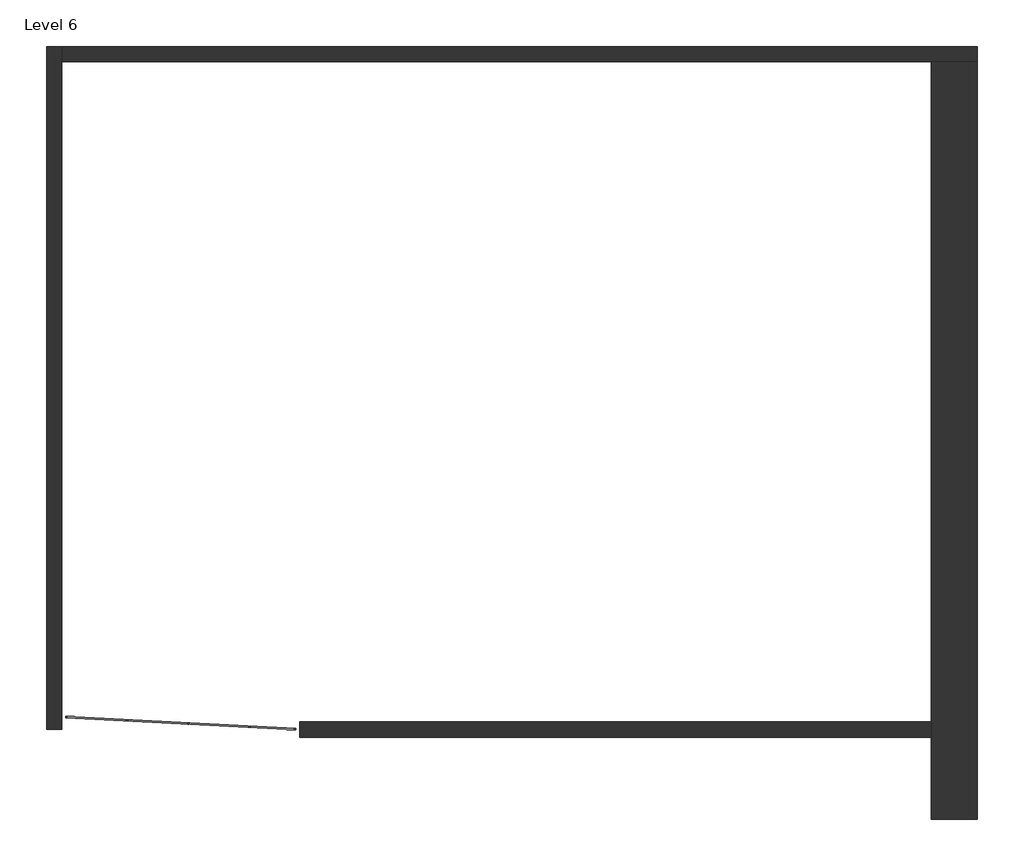
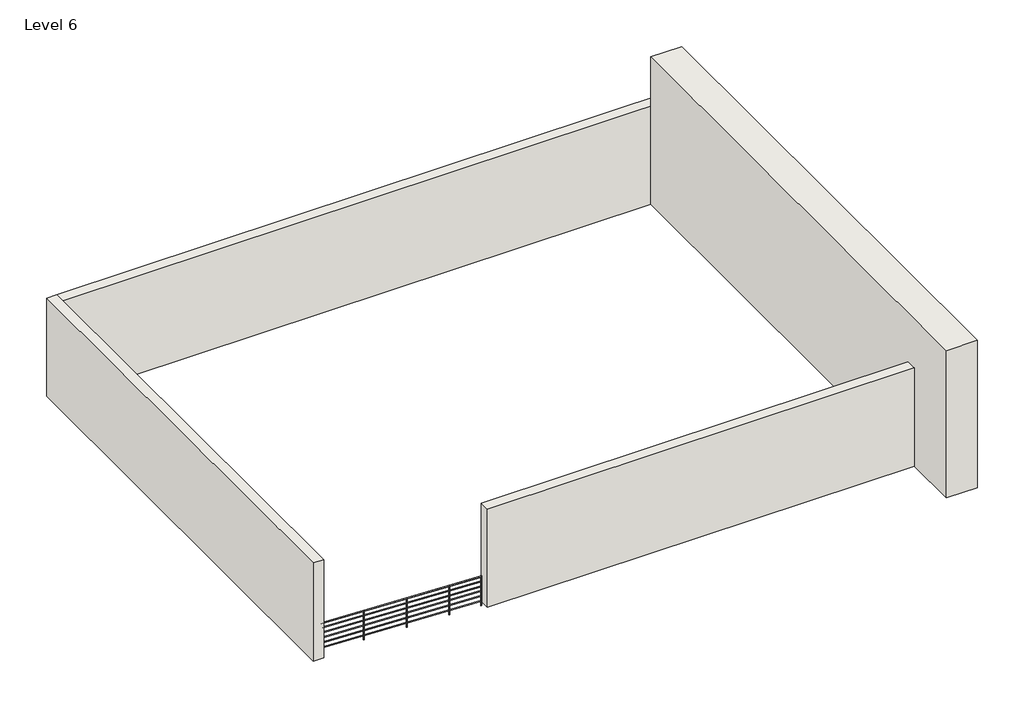
# One storey: 4 walls, 1 railing.
"""IFC4 building model written with IfcOpenShell, lengths in millimetres."""

from ifc_helpers import new_model, si_unit, point, frame, frame_2d, origin, place, context, project, spatial, polyline, circle_curve, trimmed, segment, composite_curve, outline, extrude, faceted_brep, element, save

model = new_model("IFC4")

# Units and contexts
model_context = context("Model", 3, world=origin())
ifc_project = project(units=[si_unit("LENGTHUNIT", "METRE", prefix="MILLI")], contexts=[model_context])

# Site, building, storey
site = spatial("IfcSite", under=ifc_project)
building = spatial("IfcBuilding", under=site)
storey = spatial("IfcBuildingStorey", under=building, Name="Level 6", Elevation=15240.0)

# Railing
placement = place(None, origin())
element("IfcRailing", 1, ObjectType="Handrail - Pipe", at=placement, inside=storey, context=model_context, shape_type="SweptSolid", body=[
    extrude(outline(composite_curve([segment(trimmed(circle_curve(frame_2d((0.0, 19.05)), 19.05), [point((-19.0500001, 19.05))], [point((19.05, 19.05))], False, "CARTESIAN"), True, "CONTINUOUS"), segment(trimmed(circle_curve(frame_2d((0.0, 19.05)), 19.05), [point((19.05, 19.05))], [point((-19.0500001, 19.05))], False, "CARTESIAN"), True, "CONTINUOUS")], self_intersect=False)), frame((-15001.1631562, 4736.2899368, 16764.0), z_axis=(-0.9986295347545737, 0.052335956242947373, 0.0), x_axis=(0.052335956242947373, 0.9986295347545737, 0.0)), (0.0, 0.0, 1.0), 4572.0),
    extrude(outline(composite_curve([segment(trimmed(circle_curve(frame_2d((0.0, 12.7)), 12.7), [point((12.7, 12.7))], [point((-12.7, 12.7))], False, "CARTESIAN"), True, "CONTINUOUS"), segment(trimmed(circle_curve(frame_2d((0.0, 12.7)), 12.7), [point((-12.7, 12.7))], [point((12.7, 12.7))], False, "CARTESIAN"), True, "CONTINUOUS")], self_intersect=False)), frame((-15001.1631562, 4736.2899368, 16611.6), z_axis=(-0.9986295347545737, 0.052335956242947373, 0.0), x_axis=(0.052335956242947373, 0.9986295347545737, 0.0)), (0.0, 0.0, 1.0), 4572.0),
    extrude(outline(composite_curve([segment(trimmed(circle_curve(frame_2d((0.0, 12.7)), 12.7), [point((12.7, 12.7))], [point((-12.7, 12.7))], False, "CARTESIAN"), True, "CONTINUOUS"), segment(trimmed(circle_curve(frame_2d((0.0, 12.7)), 12.7), [point((-12.7, 12.7))], [point((12.7, 12.7))], False, "CARTESIAN"), True, "CONTINUOUS")], self_intersect=False)), frame((-15001.1631562, 4736.2899368, 16459.2), z_axis=(-0.9986295347545737, 0.052335956242947373, 0.0), x_axis=(0.052335956242947373, 0.9986295347545737, 0.0)), (0.0, 0.0, 1.0), 4572.0),
    extrude(outline(composite_curve([segment(trimmed(circle_curve(frame_2d((0.0, 12.7)), 12.7), [point((12.7, 12.7))], [point((-12.7, 12.7))], False, "CARTESIAN"), True, "CONTINUOUS"), segment(trimmed(circle_curve(frame_2d((0.0, 12.7)), 12.7), [point((-12.7, 12.7))], [point((12.7, 12.7))], False, "CARTESIAN"), True, "CONTINUOUS")], self_intersect=False)), frame((-15001.1631562, 4736.2899368, 16306.8), z_axis=(-0.9986295347545737, 0.052335956242947373, 0.0), x_axis=(0.052335956242947373, 0.9986295347545737, 0.0)), (0.0, 0.0, 1.0), 4572.0),
    extrude(outline(composite_curve([segment(trimmed(circle_curve(frame_2d((0.0, 12.7)), 12.7), [point((12.7, 12.7))], [point((-12.7, 12.7))], False, "CARTESIAN"), True, "CONTINUOUS"), segment(trimmed(circle_curve(frame_2d((0.0, 12.7)), 12.7), [point((-12.7, 12.7))], [point((12.7, 12.7))], False, "CARTESIAN"), True, "CONTINUOUS")], self_intersect=False)), frame((-15001.1631562, 4736.2899368, 16154.4), z_axis=(-0.9986295347545737, 0.052335956242947373, 0.0), x_axis=(0.052335956242947373, 0.9986295347545737, 0.0)), (0.0, 0.0, 1.0), 4572.0),
    extrude(outline(composite_curve([segment(trimmed(circle_curve(frame_2d((0.0, 12.7)), 12.7), [point((12.7, 12.7))], [point((-12.7, 12.7))], False, "CARTESIAN"), True, "CONTINUOUS"), segment(trimmed(circle_curve(frame_2d((0.0, 12.7)), 12.7), [point((-12.7, 12.7))], [point((12.7, 12.7))], False, "CARTESIAN"), True, "CONTINUOUS")], self_intersect=False)), frame((-15001.1631562, 4736.2899368, 16002.0), z_axis=(-0.9986295347545737, 0.052335956242947373, 0.0), x_axis=(0.052335956242947373, 0.9986295347545737, 0.0)), (0.0, 0.0, 1.0), 4572.0),
    extrude(outline(composite_curve([segment(trimmed(circle_curve(frame_2d((-15914.3100028, 4784.1459352)), 12.7), [point((-15913.6453361, 4796.8285303))], [point((-15914.9746694, 4771.4633401))], False, "CARTESIAN"), True, "CONTINUOUS"), segment(trimmed(circle_curve(frame_2d((-15914.3100028, 4784.1459352)), 12.7), [point((-15914.9746694, 4771.4633401))], [point((-15913.6453361, 4796.8285303))], False, "CARTESIAN"), True, "CONTINUOUS")], self_intersect=False)), frame((0.0, 0.0, 15849.6), z_axis=(0.0, 0.0, 1.0), x_axis=(1.0, 0.0, 0.0)), (0.0, 0.0, 1.0), 876.3),
    extrude(outline(composite_curve([segment(trimmed(circle_curve(frame_2d((-17131.8391315, 4847.953933)), 12.7), [point((-17131.1744649, 4860.6365281))], [point((-17132.5037982, 4835.2713379))], False, "CARTESIAN"), True, "CONTINUOUS"), segment(trimmed(circle_curve(frame_2d((-17131.8391315, 4847.953933)), 12.7), [point((-17132.5037982, 4835.2713379))], [point((-17131.1744649, 4860.6365281))], False, "CARTESIAN"), True, "CONTINUOUS")], self_intersect=False)), frame((0.0, 0.0, 15849.6), z_axis=(0.0, 0.0, 1.0), x_axis=(1.0, 0.0, 0.0)), (0.0, 0.0, 1.0), 876.3),
    extrude(outline(composite_curve([segment(trimmed(circle_curve(frame_2d((-18349.3682603, 4911.7619309)), 12.7), [point((-18348.7035937, 4924.444526))], [point((-18350.032927, 4899.0793358))], False, "CARTESIAN"), True, "CONTINUOUS"), segment(trimmed(circle_curve(frame_2d((-18349.3682603, 4911.7619309)), 12.7), [point((-18350.032927, 4899.0793358))], [point((-18348.7035937, 4924.444526))], False, "CARTESIAN"), True, "CONTINUOUS")], self_intersect=False)), frame((0.0, 0.0, 15849.6), z_axis=(0.0, 0.0, 1.0), x_axis=(1.0, 0.0, 0.0)), (0.0, 0.0, 1.0), 876.3),
    extrude(outline(composite_curve([segment(trimmed(circle_curve(frame_2d((-15013.8457513, 4736.9546034)), 12.7), [point((-15013.1810846, 4749.6371985))], [point((-15014.5104179, 4724.2720083))], False, "CARTESIAN"), True, "CONTINUOUS"), segment(trimmed(circle_curve(frame_2d((-15013.8457513, 4736.9546034)), 12.7), [point((-15014.5104179, 4724.2720083))], [point((-15013.1810846, 4749.6371985))], False, "CARTESIAN"), True, "CONTINUOUS")], self_intersect=False)), frame((0.0, 0.0, 15849.6), z_axis=(0.0, 0.0, 1.0), x_axis=(1.0, 0.0, 0.0)), (0.0, 0.0, 1.0), 876.3),
    extrude(outline(composite_curve([segment(trimmed(circle_curve(frame_2d((-19554.214794, 4974.9052621)), 12.7), [point((-19553.5501274, 4987.5878572))], [point((-19554.8794606, 4962.222667))], False, "CARTESIAN"), True, "CONTINUOUS"), segment(trimmed(circle_curve(frame_2d((-19554.214794, 4974.9052621)), 12.7), [point((-19554.8794606, 4962.222667))], [point((-19553.5501274, 4987.5878572))], False, "CARTESIAN"), True, "CONTINUOUS")], self_intersect=False)), frame((0.0, 0.0, 15849.6), z_axis=(0.0, 0.0, 1.0), x_axis=(1.0, 0.0, 0.0)), (0.0, 0.0, 1.0), 876.3),
])

# Walls
element("IfcWall", 2, ObjectType="Generic - 12\" 2", at=placement, inside=storey, context=model_context, shape_type="Brep", body=[
    faceted_brep([(-19945.2572696, 18294.9189192, 15849.6), (-19945.2572696, 4731.3189192, 15849.6), (-19945.2572696, 4731.3189192, 18897.6), (-19945.2572696, 18294.9189192, 18897.6), (-19640.4572696, 18294.9189192, 15849.6), (-19640.4572696, 18294.9189192, 18897.6), (-19640.4572696, 17990.1189192, 18897.6), (-19640.4572696, 4731.3189192, 18897.6), (-19640.4572696, 4731.3189192, 15849.6), (-19640.4572696, 17990.1189192, 15849.6)], [[[0, 1, 2, 3]], [[4, 5, 6, 7, 8, 9]], [[1, 0, 4, 9, 8]], [[2, 1, 8, 7]], [[3, 2, 7, 6, 5]], [[0, 3, 5, 4]]]),
])
element("IfcWall", 3, ObjectType="Generic - 12\" 2", at=placement, inside=storey, context=model_context, shape_type="Brep", body=[
    faceted_brep([(-19640.4572696, 17990.1189192, 15849.6), (-2381.9208581, 17990.1189192, 15849.6), (-1467.5208581, 17990.1189192, 15849.6), (-1467.5208581, 17990.1189192, 18897.6), (-19640.4572696, 17990.1189192, 18897.6), (-19640.4572696, 18294.9189192, 15849.6), (-19640.4572696, 18294.9189192, 18897.6), (-1467.5208581, 18294.9189192, 18897.6), (-1467.5208581, 18294.9189192, 15849.6)], [[[0, 1, 2, 3, 4]], [[5, 6, 7, 8]], [[2, 1, 0, 5, 8]], [[4, 3, 7, 6]], [[0, 4, 6, 5]], [[3, 2, 8, 7]]]),
])
element("IfcWall", 4, ObjectType="Generic - 12\" 2", at=placement, inside=storey, context=model_context, shape_type="SweptSolid", body=[
    extrude(outline(polyline([(-14916.0572696, 4883.7189192), (-2381.9208581, 4883.7189192), (-2381.9208581, 4578.9189192), (-14916.0572696, 4578.9189192), (-14916.0572696, 4883.7189192)])), frame((0.0, 0.0, 15849.6), z_axis=(0.0, 0.0, 1.0), x_axis=(1.0, 0.0, 0.0)), (0.0, 0.0, 1.0), 3048.0),
])
element("IfcWall", 5, ObjectType="Generic - 3' 4", at=placement, inside=storey, context=model_context, shape_type="Brep", body=[
    faceted_brep([(-1467.5208581, 2947.9145816, 15849.6), (-1467.5208581, 17990.1189192, 15849.6), (-1467.5208581, 17990.1189192, 18897.6), (-1467.5208581, 17990.1189192, 20421.6), (-1467.5208581, 2947.9145816, 20421.6), (-2381.9208581, 2947.9145816, 15849.6), (-2381.9208581, 2947.9145816, 20421.6), (-2381.9208581, 17990.1189192, 20421.6), (-2381.9208581, 17990.1189192, 15849.6), (-2381.9208581, 4883.7189192, 15849.6), (-2381.9208581, 4578.9189192, 15849.6)], [[[0, 1, 2, 3, 4]], [[5, 6, 7, 8, 9, 10]], [[1, 0, 5, 10, 9, 8]], [[4, 3, 7, 6]], [[0, 4, 6, 5]], [[3, 2, 1, 8, 7]]]),
])

save(model, "model.ifc")

# Revit data of these elements
# Type "Handrail - Pipe"
#   Assembly Code = "C2010400"
#   built-in parameter 1008612 = 0.0416667 (stored number, unit not read)
#   built-in parameter 1008611 = 0.0833333 (stored number, unit not read)
#   built-in parameter 1008609 = 4 (stored number, unit not read)
#   built-in parameter 1008604 = 0.166667 (stored number, unit not read)
#   built-in parameter 1008603 = 0.166667 (stored number, unit not read)
#   Railing Height = 3' - 0"
#   built-in parameter 1008630 = 2
#   built-in parameter 1008610 = 1
#   built-in parameter 1008605 = 1
#   built-in parameter 1008618 = Baluster - Round : 1"
# Type "Generic - 12\" 2"
#   Assembly Code = "B2010"
#   Layers, outside or top first: 1' - 0" "Parking Stripe" (function 1)
# Type "Generic - 3' 4"
#   Assembly Code = "B2010"
#   Layers, outside or top first: 3' - 0" "Parking Stripe" (function 1)
# Element 1 (IfcRailing, "Handrail - Pipe")
#   built-in parameter 1008621 = 2 (stored number, unit not read)
#   Phase Created = New Construction
# Elements 2, 3, 4 (IfcWall, "Generic - 12\" 2")
#   built-in parameter 1001111 = 2' - 0"
#   Top Offset = 0' - 0"
#   Base Offset = 2' - 0"
#   Unconnected Height = 10' - 0"
#   wall height = 10' - 0"
#   Phase Created = New Construction
#   Base Constraint = Level 6
#   Materials on its faces: "Parking Stripe"
# Element 5 (IfcWall, "Generic - 3' 4")
#   built-in parameter 1001111 = 2' - 0"
#   Top Offset = 0' - 0"
#   Base Offset = 2' - 0"
#   Unconnected Height = 15' - 0"
#   wall height = 15' - 0"
#   Phase Created = New Construction
#   Base Constraint = Level 6
#   Materials on its faces: "Parking Stripe"
# Materials
#   "Parking Stripe": class "Paint", colour RGB 255 221 187, transparency 0, Cost = 0
